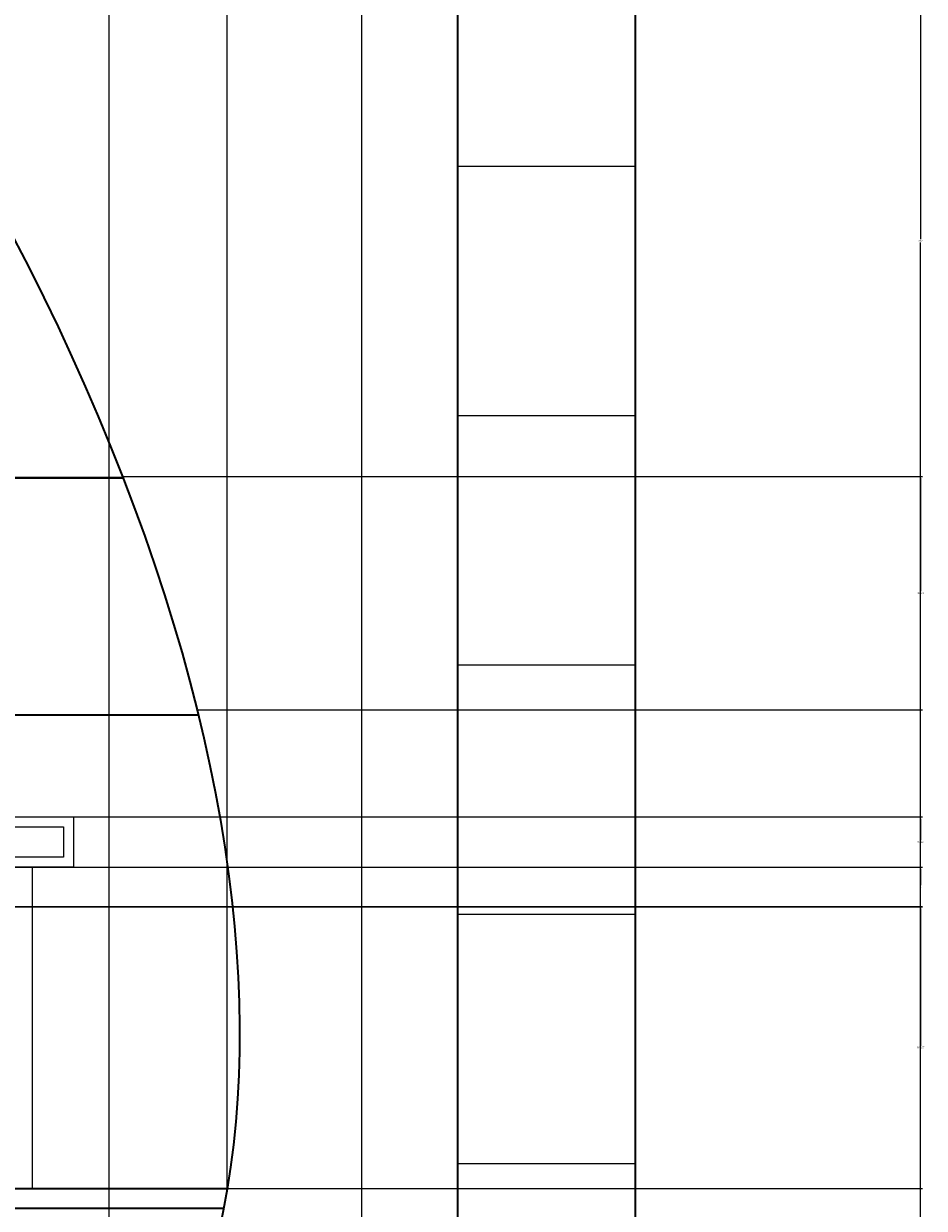
# Model space of a CAD drawing. Units: inches. Extents: x -19 to 408, y -26 to 603.
# Tile 4 of 7: x 317 to 408, y 169 to 289. Entities that reach past the tile are written whole.
import ezdxf

# ---------------------------------------------------------------- set-up
doc = ezdxf.new("R2010")
doc.units = ezdxf.units.IN
doc.header["$MEASUREMENT"] = 0
for name, color, linetype, lineweight in [('A-ANNO-DIMS', 2, 'Continuous', 18), ('A-ELEV', 7, 'Continuous', 35), ('A-GLAZ', 4, 'Continuous', 25), ('A-WALL-PATT', 8, 'Continuous', 13)]:
    doc.layers.add(name, color=color, linetype=linetype, lineweight=lineweight)
doc.styles.get("Standard").update_dxf_attribs({"font": 'arial.ttf'})
doc.dimstyles.get("Standard").update_dxf_attribs({"dimtxt": 0.18, "dimasz": 0.18, "dimexe": 0.18, "dimexo": 0.0625, "dimgap": 0.09, "dimtad": 0, "dimtih": 1, "dimtoh": 1, "dimdec": 4, "dimzin": 0, "dimdsep": 46, "dimtxsty": 'Standard', "dimcen": 0.09, "dimadec": 0, "dimazin": 0, "dimtfac": 1, "dimtdec": 4, "dimtofl": 0, "dimtmove": 0, "dimatfit": 3, "dimfxl": 1, "dimtolj": 1, "dimtzin": 0, "dimarcsym": 0})

# ---------------------------------------------------------------- blocks, each defined once
blk = doc.blocks.new('WIN-1200')
for points in [[(0, 32.56), (59.66, 32.56), (59.66, 37.64), (0, 37.64)], [(1, 33.56), (58.66, 33.56), (58.66, 36.64), (1, 36.64)]]:
    blk.add_lwpolyline(points, close=True)
for points in [[(4.17, 0), (4.17, 32.56), (55.99, 32.56), (55.99, 0)], [(8.17, 0), (8.17, 28.56), (51.99, 28.56), (51.99, 0)]]:
    blk.add_lwpolyline(points)
blk = doc.blocks.new('*D23')
at = {"layer": 'A-ANNO-DIMS', "color": 0, "lineweight": -2, "transparency": 16777216}
for p, q in [((360.63, 411.15), (407.65, 411.15)), ((407.47, 410.97), (407.47, 267.33)), ((407.47, 123.33), (407.47, 266.97)), ((360.63, 123.15), (407.65, 123.15))]:
    blk.add_line(p, q, dxfattribs=at)
at = {"layer": 'A-ANNO-DIMS', "color": 0, "transparency": 16777216}
for points in [[(407.44, 410.97), (407.5, 410.97), (407.47, 411.15)], [(407.44, 123.33), (407.5, 123.33), (407.47, 123.15)]]:
    blk.add_solid(points, dxfattribs=at)
at = {"layer": 'Defpoints', "color": 0, "transparency": 16777216}
for p in [(360.57, 411.15), (407.47, 411.15), (360.57, 123.15)]:
    blk.add_point(p, dxfattribs=at)
at = {"layer": 'A-ANNO-DIMS', "color": 0, "transparency": 16777216, "insert": (407.47, 267.15), "char_height": 0.18, "attachment_point": 5}
blk.add_mtext('\\A1;288', dxfattribs=at)
blk = doc.blocks.new('*D27')
at = {"layer": 'A-ANNO-DIMS', "color": 0, "lineweight": -2, "transparency": 16777216}
for p, q in [((288.17, 123.21), (288.17, 602.9)), ((288.35, 602.72), (324.05, 602.72)), ((360.39, 602.72), (324.69, 602.72)), ((360.57, 123.21), (360.57, 602.9))]:
    blk.add_line(p, q, dxfattribs=at)
at = {"layer": 'A-ANNO-DIMS', "color": 0, "transparency": 16777216}
for points in [[(288.35, 602.75), (288.35, 602.69), (288.17, 602.72)], [(360.39, 602.75), (360.39, 602.69), (360.57, 602.72)]]:
    blk.add_solid(points, dxfattribs=at)
at = {"layer": 'Defpoints', "color": 0, "transparency": 16777216}
for p in [(360.57, 602.72), (288.17, 123.15), (360.57, 123.15)]:
    blk.add_point(p, dxfattribs=at)
at = {"layer": 'A-ANNO-DIMS', "color": 0, "transparency": 16777216, "insert": (324.37, 602.72), "char_height": 0.18, "attachment_point": 5}
blk.add_mtext('\\A1;72.4', dxfattribs=at)
blk = doc.blocks.new('*D30')
at = {"layer": 'A-ANNO-DIMS', "color": 0, "lineweight": -2, "transparency": 16777216}
for p, q in [((360.57, 411.08), (360.57, -25.93)), ((185.52, 387.08), (185.52, -25.93)), ((185.7, -25.75), (272.59, -25.75)), ((360.39, -25.75), (273.5, -25.75))]:
    blk.add_line(p, q, dxfattribs=at)
at = {"layer": 'A-ANNO-DIMS', "color": 0, "transparency": 16777216}
for points in [[(185.7, -25.72), (185.7, -25.78), (185.52, -25.75)], [(360.39, -25.72), (360.39, -25.78), (360.57, -25.75)]]:
    blk.add_solid(points, dxfattribs=at)
at = {"layer": 'Defpoints', "color": 0, "transparency": 16777216}
for p in [(360.57, 411.15), (185.52, 387.15), (360.57, -25.75)]:
    blk.add_point(p, dxfattribs=at)
at = {"layer": 'A-ANNO-DIMS', "color": 0, "transparency": 16777216, "insert": (273.05, -25.75), "char_height": 0.18, "attachment_point": 5}
blk.add_mtext('\\A1;175.05', dxfattribs=at)
blk = doc.blocks.new('*D31')
at = {"layer": 'A-ANNO-DIMS', "color": 0, "lineweight": -2, "transparency": 16777216}
for p, q in [((326.68, 243.29), (407.65, 243.29)), ((407.47, 243.11), (407.47, 231.65)), ((407.47, 219.83), (407.47, 231.29)), ((334.23, 219.65), (407.65, 219.65))]:
    blk.add_line(p, q, dxfattribs=at)
at = {"layer": 'A-ANNO-DIMS', "color": 0, "transparency": 16777216}
for points in [[(407.44, 243.11), (407.5, 243.11), (407.47, 243.29)], [(407.44, 219.83), (407.5, 219.83), (407.47, 219.65)]]:
    blk.add_solid(points, dxfattribs=at)
at = {"layer": 'Defpoints', "color": 0, "transparency": 16777216}
for p in [(326.62, 243.29), (407.47, 243.29), (334.17, 219.65)]:
    blk.add_point(p, dxfattribs=at)
at = {"layer": 'A-ANNO-DIMS', "color": 0, "transparency": 16777216, "insert": (407.47, 231.47), "char_height": 0.18, "attachment_point": 5}
blk.add_mtext('\\A1;23.64', dxfattribs=at)
blk = doc.blocks.new('*D46')
at = {"layer": 'A-ANNO-DIMS', "color": 0, "lineweight": -2, "transparency": 16777216}
for p, q in [((337.23, 171.21), (337.23, 602.9)), ((337.41, 602.72), (348.43, 602.72)), ((360.39, 602.72), (349.36, 602.72)), ((360.57, 173.74), (360.57, 602.9))]:
    blk.add_line(p, q, dxfattribs=at)
at = {"layer": 'A-ANNO-DIMS', "color": 0, "transparency": 16777216}
for points in [[(337.41, 602.75), (337.41, 602.69), (337.23, 602.72)], [(360.39, 602.75), (360.39, 602.69), (360.57, 602.72)]]:
    blk.add_solid(points, dxfattribs=at)
at = {"layer": 'Defpoints', "color": 0, "transparency": 16777216}
for p in [(360.57, 602.72), (360.57, 173.67), (337.23, 171.15)]:
    blk.add_point(p, dxfattribs=at)
at = {"layer": 'A-ANNO-DIMS', "color": 0, "transparency": 16777216, "insert": (348.9, 602.72), "char_height": 0.18, "attachment_point": 5}
blk.add_mtext('\\A1;23.345', dxfattribs=at)
blk = doc.blocks.new('*D50')
at = {"layer": 'A-ANNO-DIMS', "color": 0, "lineweight": -2, "transparency": 16777216}
for p, q in [((104.21, 199.7), (407.65, 199.7)), ((407.47, 199.52), (407.47, 185.61)), ((407.47, 171.33), (407.47, 185.24)), ((104.21, 171.15), (407.65, 171.15))]:
    blk.add_line(p, q, dxfattribs=at)
at = {"layer": 'A-ANNO-DIMS', "color": 0, "transparency": 16777216}
for points in [[(407.44, 199.52), (407.5, 199.52), (407.47, 199.7)], [(407.44, 171.33), (407.5, 171.33), (407.47, 171.15)]]:
    blk.add_solid(points, dxfattribs=at)
at = {"layer": 'Defpoints', "color": 0, "transparency": 16777216}
for p in [(104.14, 199.7), (407.47, 199.7), (104.14, 171.15)]:
    blk.add_point(p, dxfattribs=at)
at = {"layer": 'A-ANNO-DIMS', "color": 0, "transparency": 16777216, "insert": (407.47, 185.43), "char_height": 0.18, "attachment_point": 5}
blk.add_mtext('\\A1;28.557', dxfattribs=at)
blk = doc.blocks.new('*D51')
at = {"layer": 'A-ANNO-DIMS', "color": 0, "lineweight": -2, "transparency": 16777216}
for p, q in [((108.207069, 203.703989), (407.651202, 203.703989)), ((407.471202, 203.523989), (407.471202, 201.883989)), ((407.471202, 199.883989), (407.471202, 201.523989)), ((104.207069, 199.703989), (407.651202, 199.703989))]:
    blk.add_line(p, q, dxfattribs=at)
at = {"layer": 'A-ANNO-DIMS', "color": 0, "transparency": 16777216}
for points in [[(407.441202, 203.523989), (407.501202, 203.523989), (407.471202, 203.703989)], [(407.441202, 199.883989), (407.501202, 199.883989), (407.471202, 199.703989)]]:
    blk.add_solid(points, dxfattribs=at)
at = {"layer": 'Defpoints', "color": 0, "transparency": 16777216}
for p in [(108.144569, 203.703989), (407.471202, 203.703989), (104.144569, 199.703989)]:
    blk.add_point(p, dxfattribs=at)
at = {"layer": 'A-ANNO-DIMS', "color": 0, "transparency": 16777216, "insert": (407.471202, 201.703989), "char_height": 0.18, "attachment_point": 5}
blk.add_mtext('\\A1;4', dxfattribs=at)
blk = doc.blocks.new('*D52')
at = {"layer": 'A-ANNO-DIMS', "color": 0, "lineweight": -2, "transparency": 16777216}
for p, q in [((111.87, 208.79), (407.65, 208.79)), ((407.47, 208.61), (407.47, 206.43)), ((407.47, 203.88), (407.47, 206.07)), ((111.87, 203.7), (407.65, 203.7))]:
    blk.add_line(p, q, dxfattribs=at)
at = {"layer": 'A-ANNO-DIMS', "color": 0, "transparency": 16777216}
for points in [[(407.44, 208.61), (407.5, 208.61), (407.47, 208.79)], [(407.44, 203.88), (407.5, 203.88), (407.47, 203.7)]]:
    blk.add_solid(points, dxfattribs=at)
at = {"layer": 'Defpoints', "color": 0, "transparency": 16777216}
for p in [(111.81, 208.79), (407.47, 208.79), (111.81, 203.7)]:
    blk.add_point(p, dxfattribs=at)
at = {"layer": 'A-ANNO-DIMS', "color": 0, "transparency": 16777216, "insert": (407.47, 206.25), "char_height": 0.18, "attachment_point": 5}
blk.add_mtext('\\A1;5.086', dxfattribs=at)
blk = doc.blocks.new('*D59')
at = {"layer": 'A-ANNO-DIMS', "color": 0, "lineweight": -2, "transparency": 16777216}
for p, q in [((161.15, 199.7), (407.65, 199.7)), ((407.47, 199.52), (407.47, 185.61)), ((407.47, 171.33), (407.47, 185.24)), ((161.15, 171.15), (407.65, 171.15))]:
    blk.add_line(p, q, dxfattribs=at)
at = {"layer": 'A-ANNO-DIMS', "color": 0, "transparency": 16777216}
for points in [[(407.44, 199.52), (407.5, 199.52), (407.47, 199.7)], [(407.44, 171.33), (407.5, 171.33), (407.47, 171.15)]]:
    blk.add_solid(points, dxfattribs=at)
at = {"layer": 'Defpoints', "color": 0, "transparency": 16777216}
for p in [(161.09, 199.7), (407.47, 199.7), (161.09, 171.15)]:
    blk.add_point(p, dxfattribs=at)
at = {"layer": 'A-ANNO-DIMS', "color": 0, "transparency": 16777216, "insert": (407.47, 185.43), "char_height": 0.18, "attachment_point": 5}
blk.add_mtext('\\A1;28.557', dxfattribs=at)
blk = doc.blocks.new('*D77')
at = {"layer": 'A-ANNO-DIMS', "color": 0, "lineweight": -2, "transparency": 16777216}
for p, q in [((271.51, 507.08), (271.51, -25.93)), ((325.24, 507.08), (325.24, -25.93)), ((271.69, -25.75), (297.98, -25.75)), ((325.06, -25.75), (298.77, -25.75))]:
    blk.add_line(p, q, dxfattribs=at)
at = {"layer": 'A-ANNO-DIMS', "color": 0, "transparency": 16777216}
for points in [[(271.69, -25.72), (271.69, -25.78), (271.51, -25.75)], [(325.06, -25.72), (325.06, -25.78), (325.24, -25.75)]]:
    blk.add_solid(points, dxfattribs=at)
at = {"layer": 'Defpoints', "color": 0, "transparency": 16777216}
for p in [(271.51, 507.15), (325.24, 507.15), (325.24, -25.75)]:
    blk.add_point(p, dxfattribs=at)
at = {"layer": 'A-ANNO-DIMS', "color": 0, "transparency": 16777216, "insert": (298.38, -25.75), "char_height": 0.18, "attachment_point": 5}
blk.add_mtext('\\A1;53.72', dxfattribs=at)
blk = doc.blocks.new('*D78')
at = {"layer": 'A-ANNO-DIMS', "color": 0, "lineweight": -2, "transparency": 16777216}
for p, q in [((325.24, 507.08), (325.24, -25.93)), ((350.82, 507.08), (350.82, -25.93)), ((325.42, -25.75), (337.56, -25.75)), ((350.64, -25.75), (338.49, -25.75))]:
    blk.add_line(p, q, dxfattribs=at)
at = {"layer": 'A-ANNO-DIMS', "color": 0, "transparency": 16777216}
for points in [[(325.42, -25.72), (325.42, -25.78), (325.24, -25.75)], [(350.64, -25.72), (350.64, -25.78), (350.82, -25.75)]]:
    blk.add_solid(points, dxfattribs=at)
at = {"layer": 'Defpoints', "color": 0, "transparency": 16777216}
for p in [(325.24, 507.15), (350.82, 507.15), (350.82, -25.75)]:
    blk.add_point(p, dxfattribs=at)
at = {"layer": 'A-ANNO-DIMS', "color": 0, "transparency": 16777216, "insert": (338.03, -25.75), "char_height": 0.18, "attachment_point": 5}
blk.add_mtext('\\A1;25.584', dxfattribs=at)

msp = doc.modelspace()

# ---------------------------------------------------------------- linework, layer by layer
at = {"layer": 'A-ELEV'}
for p, q in [((360.5712, 123.1472), (360.5712, 483.1472)), ((378.5712, 123.1472), (378.5712, 483.1472)), ((326.6715, 243.1472), (98.524, 243.1472)), ((98.524, 243.1472), (326.6715, 243.1472)), ((36.5712, 219.1472), (334.2819, 219.1472)), ((36.5712, 171.1472), (337.2261, 171.1472)), ((36.5712, 169.1472), (336.868, 169.1472))]:
    msp.add_line(p, q, dxfattribs=at)
at = {"layer": 'A-ELEV', "extrusion": (0, 0, -1)}
msp.add_ellipse((217.8094, 257.6617), major_axis=(99.7631, -123.1178), ratio=0.55109141, start_param=3.84421936, end_param=6.63412911, dxfattribs=at)
at = {"layer": 'A-WALL-PATT'}
for p, q in [((360.5712, 274.7262), (378.5712, 274.7262)), ((360.5712, 249.463), (378.5712, 249.463)), ((360.5712, 224.1999), (378.5712, 224.1999)), ((360.5712, 198.9367), (378.5712, 198.9367)), ((360.5712, 173.6735), (378.5712, 173.6735))]:
    msp.add_line(p, q, dxfattribs=at)

# ---------------------------------------------------------------- block references
at = {"layer": 'A-GLAZ', "extrusion": (0, 0, -1), "zscale": -1}
msp.add_blockref('WIN-1200', (-321.6443, 171.147), dxfattribs=at)

# ---------------------------------------------------------------- dimensions: what is measured, and where the dimension line sits
at = {"layer": 'A-ANNO-DIMS'}
for base, p1, p2, override, picture, middle in [((360.5712, 602.7184), (288.1664, 123.1472), (360.5712, 123.1472), {"dimdec": 1, "dimlfac": 1, "dimrnd": 0, "dimzin": 0, "dimdsep": 46, "dimlunit": 2}, '*D27', (324.3688, 602.7184)), ((360.5712, 602.7184), (337.2261, 171.1472), (360.5712, 173.6735), {"dimdec": 3, "dimlfac": 1, "dimrnd": 0, "dimzin": 0, "dimdsep": 46, "dimlunit": 2}, '*D46', (348.8986, 602.7184)), ((325.2366, -25.7528), (271.514, 507.1472), (325.2366, 507.1472), {"dimdec": 2, "dimlfac": 1, "dimrnd": 0, "dimzin": 0, "dimdsep": 46, "dimlunit": 2}, '*D77', (298.3753, -25.7528)), ((350.8209, -25.7528), (325.2366, 507.1472), (350.8209, 507.1472), {"dimdec": 3, "dimlfac": 1, "dimrnd": 0, "dimzin": 0, "dimdsep": 46, "dimlunit": 2}, '*D78', (338.0288, -25.7528)), ((360.5712, -25.7528), (185.5212, 387.1472), (360.5712, 411.1472), {"dimdec": 2, "dimlfac": 1, "dimrnd": 0, "dimzin": 0, "dimdsep": 46, "dimlunit": 2}, '*D30', (273.0462, -25.7528))]:
    dim = msp.add_linear_dim(base=base, p1=p1, p2=p2, dimstyle='Standard', override=override, dxfattribs=at)
    dim.commit()
    dim.dimension.update_dxf_attribs({"geometry": picture, "text_midpoint": middle})
for base, p1, p2, override, picture, middle in [((407.4712, 411.1472), (360.5712, 123.1472), (360.5712, 411.1472), {"dimdec": 0, "dimlfac": 1, "dimrnd": 0, "dimzin": 0, "dimdsep": 46, "dimlunit": 2}, '*D23', (407.4712, 267.1472)), ((407.4712, 243.2883), (334.169, 219.6501), (326.6167, 243.2883), {"dimdec": 2, "dimlfac": 1, "dimrnd": 0, "dimzin": 0, "dimdsep": 46, "dimlunit": 2}, '*D31', (407.4712, 231.4692)), ((407.4712, 208.7903), (111.8091, 203.704), (111.8091, 208.7903), {"dimdec": 3, "dimlfac": 1, "dimrnd": 0, "dimzin": 0, "dimdsep": 46, "dimlunit": 2}, '*D52', (407.4712, 206.2471)), ((407.4712, 203.704), (104.1446, 199.704), (108.1446, 203.704), {"dimdec": 0, "dimlfac": 1, "dimrnd": 0, "dimzin": 0, "dimdsep": 46, "dimlunit": 2}, '*D51', (407.4712, 201.704)), ((407.4712, 199.704), (104.1446, 171.1472), (104.1446, 199.704), {"dimdec": 3, "dimlfac": 1, "dimrnd": 0, "dimzin": 0, "dimdsep": 46, "dimlunit": 2}, '*D50', (407.4712, 185.4256)), ((407.4712, 199.704), (161.088, 171.1472), (161.088, 199.704), {"dimdec": 3, "dimlfac": 1, "dimrnd": 0, "dimzin": 0, "dimdsep": 46, "dimlunit": 2}, '*D59', (407.4712, 185.4256))]:
    dim = msp.add_linear_dim(base=base, p1=p1, p2=p2, angle=90, dimstyle='Standard', override=override, dxfattribs=at)
    dim.commit()
    dim.dimension.update_dxf_attribs({"geometry": picture, "text_midpoint": middle})

doc.saveas('drawing.dxf')
